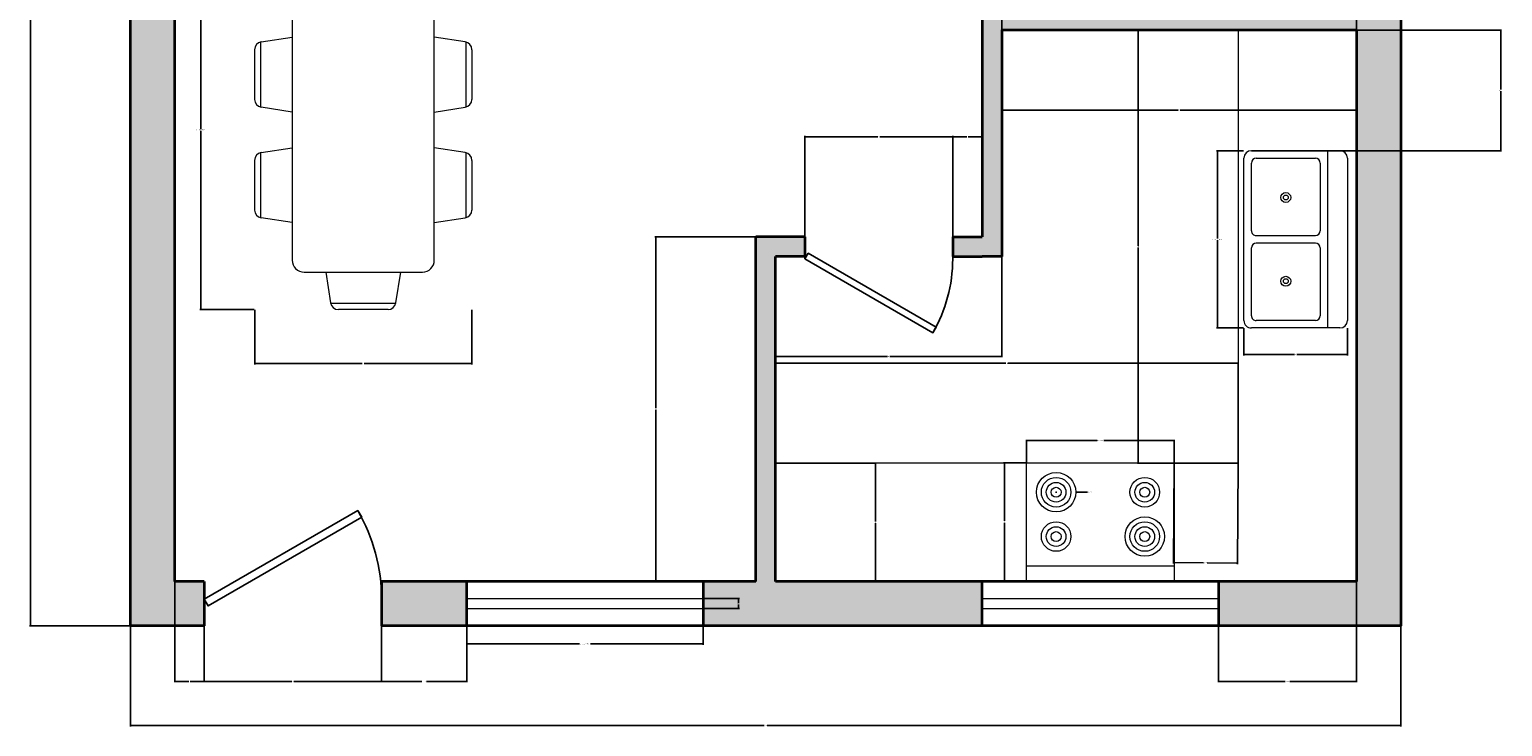
# Model space of a CAD drawing. Units: inches. Extents: x 1984 to 2284, y 2002 to 2421.
# Tile 1 of 4: x 1984 to 2284, y 2002 to 2144. Entities that reach past the tile are written whole.
import ezdxf

# ---------------------------------------------------------------- set-up
doc = ezdxf.new("R2010")
doc.units = ezdxf.units.IN
for name, color, linetype, lineweight in [('A-ANNO-DIMS', 2, 'Continuous', 18), ('A-DOOR', 3, 'Continuous', 25), ('A-EQPM', 9, 'Continuous', 18), ('A-FLOR-CASE', 9, 'Continuous', 20), ('A-FLOR-FIXT', 8, 'Continuous', 18), ('A-FURN', 8, 'Continuous', 18), ('A-GLAZ', 4, 'Continuous', 18), ('A-WALL', 7, 'Continuous', 35)]:
    doc.layers.add(name, color=color, linetype=linetype, lineweight=lineweight)
doc.layers.add('A-WALL-PATT', color=18, linetype='Continuous', lineweight=13, true_color=0x000000)
doc.styles.get("Standard").update_dxf_attribs({"font": 'arial.ttf'})
doc.dimstyles.get("Standard").update_dxf_attribs({"dimtxt": 0.18, "dimasz": 0.18, "dimexe": 0.18, "dimexo": 0.0625, "dimgap": 0.09, "dimtad": 0, "dimtih": 1, "dimtoh": 1, "dimdec": 4, "dimzin": 0, "dimdsep": 46, "dimtxsty": 'Standard', "dimcen": 0.09, "dimadec": 0, "dimazin": 0, "dimtfac": 1, "dimtdec": 4, "dimtofl": 0, "dimtmove": 0, "dimatfit": 3, "dimfxl": 1, "dimtolj": 1, "dimtzin": 0, "dimarcsym": 0})

# ---------------------------------------------------------------- blocks, each defined once
blk = doc.blocks.new('Range-Oven - 30 in top')
blk.add_line((0, -3), (30, -3))
blk.add_lwpolyline([(0, -24), (0, 0), (30, 0), (30, -24)], close=True)
for centre, radius in [((6, -9), 4), ((6, -9), 3), ((6, -9), 2), ((6, -9), 1), ((24, -9), 3), ((24, -9), 2), ((24, -9), 1), ((24, -18), 4), ((6, -18), 3), ((6, -18), 2), ((6, -18), 1), ((24, -18), 3), ((24, -18), 2), ((24, -18), 1)]:
    blk.add_circle(centre, radius)
blk = doc.blocks.new('Sink-double - 36 in top')
for p, q in [((-18, -4), (18, -4)), ((-0.75, -18.5), (-0.75, -6.5)), ((0.75, -6.5), (0.75, -18.5))]:
    blk.add_line(p, q)
for points in [[(-16.5, 0), (16.5, 0)], [(-18, -19.5), (-18, -1.5)], [(18, -1.5), (18, -19.5)], [(-15.5, -5.5), (-1.75, -5.5)], [(1.75, -5.5), (15.5, -5.5)], [(-16.5, -18.5), (-16.5, -6.5)], [(16.5, -6.5), (16.5, -18.5)], [(-1.75, -19.5), (-15.5, -19.5)], [(15.5, -19.5), (1.75, -19.5)], [(16.5, -21), (-16.5, -21)]]:
    blk.add_lwpolyline(points)
for centre, radius in [((-8.5, -12.5), 1), ((8.5, -12.5), 1), ((-8.5, -12.5), 0.5), ((8.5, -12.5), 0.5)]:
    blk.add_circle(centre, radius)
for centre, radius, start, end in [((-16.5, -1.5), 1.5, 90, 180), ((16.5, -1.5), 1.5, 0, 90), ((-15.5, -6.5), 1, 90, 180), ((-1.75, -6.5), 1, 0, 90), ((1.75, -6.5), 1, 90, 180), ((15.5, -6.5), 1, 0, 90), ((-16.5, -19.5), 1.5, 180, 270), ((-15.5, -18.5), 1, 180, 270), ((-1.75, -18.5), 1, 270, 0), ((1.75, -18.5), 1, 180, 270), ((15.5, -18.5), 1, 270, 0), ((16.5, -19.5), 1.5, 270, 0)]:
    blk.add_arc(centre, radius, start, end)
blk = doc.blocks.new('Dining Set - 36 x 72 in.')
for p, q in [((-20.29, 27.5), (-7.71, 27.5)), ((7.71, 27.5), (20.29, 27.5)), ((-22.26, 25.81), (-23.48, 18)), ((-22.23, 26), (-5.76, 26)), ((-4.52, 18), (-5.74, 25.81)), ((5.74, 25.81), (4.52, 18)), ((5.77, 26), (22.24, 26)), ((23.48, 18), (22.26, 25.81)), ((-36, 15), (-36, -15)), ((33, 18), (-33, 18)), ((36, -15), (36, 15)), ((-44, 8.23), (-44, -8.24)), ((-43.81, 8.26), (-36, 9.48)), ((43.81, 8.26), (36, 9.48)), ((44, 8.23), (44, -8.24)), ((-45.5, 6.29), (-45.5, -6.29)), ((45.5, 6.29), (45.5, -6.29)), ((-36, -9.48), (-43.81, -8.26)), ((36, -9.48), (43.81, -8.26)), ((-33, -18), (33, -18)), ((-22.26, -25.81), (-23.48, -18)), ((-4.52, -18), (-5.74, -25.81)), ((5.74, -25.81), (4.52, -18)), ((23.48, -18), (22.26, -25.81)), ((-22.23, -26), (-5.76, -26)), ((5.77, -26), (22.24, -26)), ((-20.29, -27.5), (-7.71, -27.5)), ((7.71, -27.5), (20.29, -27.5))]:
    blk.add_line(p, q)
for centre, radius, start, end in [((-20.29, 25.5), 2, 90, 171.1198), ((-7.71, 25.5), 2, 8.881, 90), ((7.71, 25.5), 2, 90, 171.1198), ((20.29, 25.5), 2, 8.881, 90), ((-33, 15), 3, 90, 180), ((33, 15), 3, 0, 90), ((-43.5, 6.29), 2, 98.8806, 180), ((43.5, 6.29), 2, 0, 81.1194), ((-43.5, -6.29), 2, 180, 261.1194), ((43.5, -6.29), 2, 278.8806, 0), ((-33, -15), 3, 180, 270), ((33, -15), 3, 270, 0), ((-20.29, -25.5), 2, 188.8802, 270), ((-7.71, -25.5), 2, 270, 351.1191), ((7.71, -25.5), 2, 188.8802, 270), ((20.29, -25.5), 2, 270, 351.1191)]:
    blk.add_arc(centre, radius, start, end)
blk = doc.blocks.new('*U10')
for p, q in [((0, 0), (0, -6)), ((40, 0), (40, -6))]:
    blk.add_line(p, q)
blk.add_lwpolyline([(0, 0), (34.64, 20), (35.52, 18.48), (0.87, -1.52)], close=True)
blk.add_arc((0, 0), 40, 0, 30)
blk = doc.blocks.new('*U11')
for p, q in [((0, 0), (0, 6)), ((40, 0), (40, 6))]:
    blk.add_line(p, q)
blk.add_lwpolyline([(0, 0), (34.64, -20), (35.52, -18.48), (0.87, 1.52)], close=True)
blk.add_arc((0, 0), 40, 330, 0)
blk = doc.blocks.new('GLAZING-48IN')
for p, q in [((0, 2), (48, 2)), ((0, 0), (48, 0))]:
    blk.add_line(p, q)
blk = doc.blocks.new('*D17')
at = {"layer": 'A-ANNO-DIMS', "color": 0, "lineweight": -2, "transparency": 16777216}
for p, q in [((2073.18, 2026.35), (2073.18, 2019.03)), ((2121.18, 2026.35), (2121.18, 2019.03)), ((2073.36, 2019.21), (2096.06, 2019.21)), ((2121, 2019.21), (2098.3, 2019.21))]:
    blk.add_line(p, q, dxfattribs=at)
at = {"layer": 'A-ANNO-DIMS', "color": 0, "transparency": 16777216}
for points in [[(2073.36, 2019.24), (2073.36, 2019.18), (2073.18, 2019.21)], [(2121, 2019.24), (2121, 2019.18), (2121.18, 2019.21)]]:
    blk.add_solid(points, dxfattribs=at)
at = {"layer": 'Defpoints', "color": 0, "transparency": 16777216}
for p in [(2073.18, 2026.41), (2121.18, 2026.41), (2121.18, 2019.21)]:
    blk.add_point(p, dxfattribs=at)
at = {"layer": 'A-ANNO-DIMS', "color": 0, "transparency": 16777216, "insert": (2097.18, 2019.21), "char_height": 0.18, "attachment_point": 5}
blk.add_mtext('\\A1;WINDOW 48 TYP.', dxfattribs=at)
blk = doc.blocks.new('*D18')
at = {"layer": 'A-ANNO-DIMS', "color": 0, "lineweight": -2, "transparency": 16777216}
for p, q in [((2121.24, 2028.41), (2128.56, 2028.41)), ((2121.24, 2026.41), (2128.56, 2026.41)), ((2128.38, 2028.23), (2128.38, 2027.59)), ((2128.38, 2026.59), (2128.38, 2027.23))]:
    blk.add_line(p, q, dxfattribs=at)
at = {"layer": 'A-ANNO-DIMS', "color": 0, "transparency": 16777216}
for points in [[(2128.35, 2028.23), (2128.41, 2028.23), (2128.38, 2028.41)], [(2128.35, 2026.59), (2128.41, 2026.59), (2128.38, 2026.41)]]:
    blk.add_solid(points, dxfattribs=at)
at = {"layer": 'Defpoints', "color": 0, "transparency": 16777216}
for p in [(2121.18, 2028.41), (2121.18, 2026.41), (2128.38, 2028.41)]:
    blk.add_point(p, dxfattribs=at)
at = {"layer": 'A-ANNO-DIMS', "color": 0, "transparency": 16777216, "insert": (2128.38, 2027.41), "char_height": 0.18, "attachment_point": 5}
blk.add_mtext('\\A1;2 TYP.', dxfattribs=at)
blk = doc.blocks.new('*D35')
at = {"layer": 'A-ANNO-DIMS', "color": 0, "lineweight": -2, "transparency": 16777216}
for p, q in [((2186.9, 2056.08), (2186.9, 2060.7)), ((2187.08, 2060.52), (2201.2, 2060.52)), ((2216.72, 2060.52), (2202.59, 2060.52)), ((2216.9, 2056.08), (2216.9, 2060.7))]:
    blk.add_line(p, q, dxfattribs=at)
at = {"layer": 'A-ANNO-DIMS', "color": 0, "transparency": 16777216}
for points in [[(2187.08, 2060.55), (2187.08, 2060.49), (2186.9, 2060.52)], [(2216.72, 2060.55), (2216.72, 2060.49), (2216.9, 2060.52)]]:
    blk.add_solid(points, dxfattribs=at)
at = {"layer": 'Defpoints', "color": 0, "transparency": 16777216}
for p in [(2186.9, 2060.52), (2186.9, 2056.02), (2216.9, 2056.02)]:
    blk.add_point(p, dxfattribs=at)
at = {"layer": 'A-ANNO-DIMS', "color": 0, "transparency": 16777216, "insert": (2201.9, 2060.52), "char_height": 0.18, "attachment_point": 5}
blk.add_mtext('\\A1;RANGE 30', dxfattribs=at)
blk = doc.blocks.new('*D36')
at = {"layer": 'A-ANNO-DIMS', "color": 0, "lineweight": -2, "transparency": 16777216}
for p, q in [((2186.83, 2056.02), (2182.22, 2056.02)), ((2182.4, 2055.84), (2182.4, 2044.2)), ((2182.4, 2032.2), (2182.4, 2043.84)), ((2186.83, 2032.02), (2182.22, 2032.02))]:
    blk.add_line(p, q, dxfattribs=at)
at = {"layer": 'A-ANNO-DIMS', "color": 0, "transparency": 16777216}
for points in [[(2182.37, 2055.84), (2182.43, 2055.84), (2182.4, 2056.02)], [(2182.37, 2032.2), (2182.43, 2032.2), (2182.4, 2032.02)]]:
    blk.add_solid(points, dxfattribs=at)
at = {"layer": 'Defpoints', "color": 0, "transparency": 16777216}
for p in [(2186.9, 2056.02), (2182.4, 2032.02), (2186.9, 2032.02)]:
    blk.add_point(p, dxfattribs=at)
at = {"layer": 'A-ANNO-DIMS', "color": 0, "transparency": 16777216, "insert": (2182.4, 2044.02), "char_height": 0.18, "attachment_point": 5}
blk.add_mtext('\\A1;24', dxfattribs=at)
blk = doc.blocks.new('*D37')
at = {"layer": 'A-ANNO-DIMS', "color": 0, "lineweight": -2, "transparency": 16777216}
for p, q in [((2230.98, 2119.39), (2225.46, 2119.39)), ((2225.64, 2119.21), (2225.64, 2101.57)), ((2225.64, 2083.57), (2225.64, 2101.2)), ((2230.98, 2083.39), (2225.46, 2083.39))]:
    blk.add_line(p, q, dxfattribs=at)
at = {"layer": 'A-ANNO-DIMS', "color": 0, "transparency": 16777216}
for points in [[(2225.61, 2119.21), (2225.67, 2119.21), (2225.64, 2119.39)], [(2225.61, 2083.57), (2225.67, 2083.57), (2225.64, 2083.39)]]:
    blk.add_solid(points, dxfattribs=at)
at = {"layer": 'Defpoints', "color": 0, "transparency": 16777216}
for p in [(2231.04, 2119.39), (2225.64, 2083.39), (2231.04, 2083.39)]:
    blk.add_point(p, dxfattribs=at)
at = {"layer": 'A-ANNO-DIMS', "color": 0, "transparency": 16777216, "insert": (2225.64, 2101.39), "char_height": 0.18, "attachment_point": 5}
blk.add_mtext('\\A1;DOUBLE SINK 36', dxfattribs=at)
blk = doc.blocks.new('*D38')
at = {"layer": 'A-ANNO-DIMS', "color": 0, "lineweight": -2, "transparency": 16777216}
for p, q in [((2231.04, 2083.32), (2231.04, 2077.81)), ((2252.04, 2083.32), (2252.04, 2077.81)), ((2231.22, 2077.99), (2241.34, 2077.99)), ((2251.86, 2077.99), (2241.75, 2077.99))]:
    blk.add_line(p, q, dxfattribs=at)
at = {"layer": 'A-ANNO-DIMS', "color": 0, "transparency": 16777216}
for points in [[(2231.22, 2078.02), (2231.22, 2077.96), (2231.04, 2077.99)], [(2251.86, 2078.02), (2251.86, 2077.96), (2252.04, 2077.99)]]:
    blk.add_solid(points, dxfattribs=at)
at = {"layer": 'Defpoints', "color": 0, "transparency": 16777216}
for p in [(2231.04, 2083.39), (2252.04, 2083.39), (2252.04, 2077.99)]:
    blk.add_point(p, dxfattribs=at)
at = {"layer": 'A-ANNO-DIMS', "color": 0, "transparency": 16777216, "insert": (2241.54, 2077.99), "char_height": 0.18, "attachment_point": 5}
blk.add_mtext('\\A1;21', dxfattribs=at)
blk = doc.blocks.new('*D39')
at = {"layer": 'A-ANNO-DIMS', "color": 0, "lineweight": -2, "transparency": 16777216}
for p, q in [((2030.05, 2160.11), (2018.99, 2160.11)), ((2019.17, 2159.93), (2019.17, 2123.8)), ((2019.17, 2087.31), (2019.17, 2123.44)), ((2030.05, 2087.13), (2018.99, 2087.13))]:
    blk.add_line(p, q, dxfattribs=at)
at = {"layer": 'A-ANNO-DIMS', "color": 0, "transparency": 16777216}
for points in [[(2019.14, 2159.93), (2019.2, 2159.93), (2019.17, 2160.11)], [(2019.14, 2087.31), (2019.2, 2087.31), (2019.17, 2087.13)]]:
    blk.add_solid(points, dxfattribs=at)
at = {"layer": 'Defpoints', "color": 0, "transparency": 16777216}
for p in [(2030.12, 2160.11), (2019.17, 2087.13), (2030.12, 2087.13)]:
    blk.add_point(p, dxfattribs=at)
at = {"layer": 'A-ANNO-DIMS', "color": 0, "transparency": 16777216, "insert": (2019.17, 2123.62), "char_height": 0.18, "attachment_point": 5}
blk.add_mtext('\\A1;DINING SET 73', dxfattribs=at)
blk = doc.blocks.new('*D40')
at = {"layer": 'A-ANNO-DIMS', "color": 0, "lineweight": -2, "transparency": 16777216}
for p, q in [((2030.12, 2087.07), (2030.12, 2076)), ((2074.23, 2087.07), (2074.23, 2076)), ((2030.3, 2076.18), (2051.95, 2076.18)), ((2074.05, 2076.18), (2052.39, 2076.18))]:
    blk.add_line(p, q, dxfattribs=at)
at = {"layer": 'A-ANNO-DIMS', "color": 0, "transparency": 16777216}
for points in [[(2030.3, 2076.21), (2030.3, 2076.15), (2030.12, 2076.18)], [(2074.05, 2076.21), (2074.05, 2076.15), (2074.23, 2076.18)]]:
    blk.add_solid(points, dxfattribs=at)
at = {"layer": 'Defpoints', "color": 0, "transparency": 16777216}
for p in [(2030.12, 2087.13), (2074.23, 2087.13), (2074.23, 2076.18)]:
    blk.add_point(p, dxfattribs=at)
at = {"layer": 'A-ANNO-DIMS', "color": 0, "transparency": 16777216, "insert": (2052.17, 2076.18), "char_height": 0.18, "attachment_point": 5}
blk.add_mtext('\\A1;44', dxfattribs=at)
blk = doc.blocks.new('*D41')
at = {"layer": 'A-ANNO-DIMS', "color": 0, "lineweight": -2, "transparency": 16777216}
for p, q in [((2004.89, 2022.85), (2004.89, 2002.43)), ((2262.89, 2022.85), (2262.89, 2002.43)), ((2005.07, 2002.61), (2133.59, 2002.61)), ((2262.71, 2002.61), (2134.18, 2002.61))]:
    blk.add_line(p, q, dxfattribs=at)
at = {"layer": 'A-ANNO-DIMS', "color": 0, "transparency": 16777216}
for points in [[(2005.07, 2002.64), (2005.07, 2002.58), (2004.89, 2002.61)], [(2262.71, 2002.64), (2262.71, 2002.58), (2262.89, 2002.61)]]:
    blk.add_solid(points, dxfattribs=at)
at = {"layer": 'Defpoints', "color": 0, "transparency": 16777216}
for p in [(2004.89, 2022.91), (2262.89, 2022.91), (2262.89, 2002.61)]:
    blk.add_point(p, dxfattribs=at)
at = {"layer": 'A-ANNO-DIMS', "color": 0, "transparency": 16777216, "insert": (2133.89, 2002.61), "char_height": 0.18, "attachment_point": 5}
blk.add_mtext('\\A1;258', dxfattribs=at)
blk = doc.blocks.new('*D42')
at = {"layer": 'A-ANNO-DIMS', "color": 0, "lineweight": -2, "transparency": 16777216}
for p, q in [((2004.82, 2400.91), (1984.41, 2400.91)), ((1984.59, 2400.73), (1984.59, 2212.09)), ((1984.59, 2023.09), (1984.59, 2211.73)), ((2004.82, 2022.91), (1984.41, 2022.91))]:
    blk.add_line(p, q, dxfattribs=at)
at = {"layer": 'A-ANNO-DIMS', "color": 0, "transparency": 16777216}
for points in [[(1984.56, 2400.73), (1984.62, 2400.73), (1984.59, 2400.91)], [(1984.56, 2023.09), (1984.62, 2023.09), (1984.59, 2022.91)]]:
    blk.add_solid(points, dxfattribs=at)
at = {"layer": 'Defpoints', "color": 0, "transparency": 16777216}
for p in [(1984.59, 2400.91), (2004.89, 2400.91), (2004.89, 2022.91)]:
    blk.add_point(p, dxfattribs=at)
at = {"layer": 'A-ANNO-DIMS', "color": 0, "transparency": 16777216, "insert": (1984.59, 2211.91), "char_height": 0.18, "attachment_point": 5}
blk.add_mtext('\\A1;378', dxfattribs=at)
blk = doc.blocks.new('*D53')
at = {"layer": 'A-ANNO-DIMS', "color": 0, "lineweight": -2, "transparency": 16777216}
for p, q in [((2229.82, 2143.91), (2209.41, 2143.91)), ((2209.59, 2143.73), (2209.59, 2100.09)), ((2209.59, 2056.09), (2209.59, 2099.73)), ((2229.82, 2055.91), (2209.41, 2055.91))]:
    blk.add_line(p, q, dxfattribs=at)
at = {"layer": 'A-ANNO-DIMS', "color": 0, "transparency": 16777216}
for points in [[(2209.56, 2143.73), (2209.62, 2143.73), (2209.59, 2143.91)], [(2209.56, 2056.09), (2209.62, 2056.09), (2209.59, 2055.91)]]:
    blk.add_solid(points, dxfattribs=at)
at = {"layer": 'Defpoints', "color": 0, "transparency": 16777216}
for p in [(2209.59, 2143.91), (2229.89, 2143.91), (2229.89, 2055.91)]:
    blk.add_point(p, dxfattribs=at)
at = {"layer": 'A-ANNO-DIMS', "color": 0, "transparency": 16777216, "insert": (2209.59, 2099.91), "char_height": 0.18, "attachment_point": 5}
blk.add_mtext('\\A1;88', dxfattribs=at)
blk = doc.blocks.new('*D54')
at = {"layer": 'A-ANNO-DIMS', "color": 0, "lineweight": -2, "transparency": 16777216}
for p, q in [((2181.89, 2147.85), (2181.89, 2127.43)), ((2253.89, 2147.85), (2253.89, 2127.43)), ((2182.07, 2127.61), (2217.67, 2127.61)), ((2253.71, 2127.61), (2218.1, 2127.61))]:
    blk.add_line(p, q, dxfattribs=at)
at = {"layer": 'A-ANNO-DIMS', "color": 0, "transparency": 16777216}
for points in [[(2182.07, 2127.64), (2182.07, 2127.58), (2181.89, 2127.61)], [(2253.71, 2127.64), (2253.71, 2127.58), (2253.89, 2127.61)]]:
    blk.add_solid(points, dxfattribs=at)
at = {"layer": 'Defpoints', "color": 0, "transparency": 16777216}
for p in [(2181.89, 2147.91), (2253.89, 2147.91), (2181.89, 2127.61)]:
    blk.add_point(p, dxfattribs=at)
at = {"layer": 'A-ANNO-DIMS', "color": 0, "transparency": 16777216, "insert": (2217.89, 2127.61), "char_height": 0.18, "attachment_point": 5}
blk.add_mtext('\\A1;72', dxfattribs=at)
blk = doc.blocks.new('*D55')
at = {"layer": 'A-ANNO-DIMS', "color": 0, "lineweight": -2, "transparency": 16777216}
for p, q in [((2131.82, 2101.91), (2111.41, 2101.91)), ((2111.59, 2101.73), (2111.59, 2067.09)), ((2111.59, 2032.09), (2111.59, 2066.73)), ((2131.82, 2031.91), (2111.41, 2031.91))]:
    blk.add_line(p, q, dxfattribs=at)
at = {"layer": 'A-ANNO-DIMS', "color": 0, "transparency": 16777216}
for points in [[(2111.56, 2101.73), (2111.62, 2101.73), (2111.59, 2101.91)], [(2111.56, 2032.09), (2111.62, 2032.09), (2111.59, 2031.91)]]:
    blk.add_solid(points, dxfattribs=at)
at = {"layer": 'Defpoints', "color": 0, "transparency": 16777216}
for p in [(2111.59, 2101.91), (2131.89, 2101.91), (2131.89, 2031.91)]:
    blk.add_point(p, dxfattribs=at)
at = {"layer": 'A-ANNO-DIMS', "color": 0, "transparency": 16777216, "insert": (2111.59, 2066.91), "char_height": 0.18, "attachment_point": 5}
blk.add_mtext('\\A1;70', dxfattribs=at)
blk = doc.blocks.new('*D56')
at = {"layer": 'A-ANNO-DIMS', "color": 0, "lineweight": -2, "transparency": 16777216}
for p, q in [((2135.89, 2097.85), (2135.89, 2077.43)), ((2181.89, 2097.85), (2181.89, 2077.43)), ((2136.07, 2077.61), (2158.66, 2077.61)), ((2181.71, 2077.61), (2159.11, 2077.61))]:
    blk.add_line(p, q, dxfattribs=at)
at = {"layer": 'A-ANNO-DIMS', "color": 0, "transparency": 16777216}
for points in [[(2136.07, 2077.64), (2136.07, 2077.58), (2135.89, 2077.61)], [(2181.71, 2077.64), (2181.71, 2077.58), (2181.89, 2077.61)]]:
    blk.add_solid(points, dxfattribs=at)
at = {"layer": 'Defpoints', "color": 0, "transparency": 16777216}
for p in [(2135.89, 2097.91), (2181.89, 2097.91), (2135.89, 2077.61)]:
    blk.add_point(p, dxfattribs=at)
at = {"layer": 'A-ANNO-DIMS', "color": 0, "transparency": 16777216, "insert": (2158.89, 2077.61), "char_height": 0.18, "attachment_point": 5}
blk.add_mtext('\\A1;46', dxfattribs=at)
blk = doc.blocks.new('*D57')
at = {"layer": 'A-ANNO-DIMS', "color": 0, "lineweight": -2, "transparency": 16777216}
for p, q in [((2019.89, 2031.85), (2019.89, 2011.43)), ((2055.89, 2031.85), (2055.89, 2011.43)), ((2020.07, 2011.61), (2037.67, 2011.61)), ((2055.71, 2011.61), (2038.1, 2011.61))]:
    blk.add_line(p, q, dxfattribs=at)
at = {"layer": 'A-ANNO-DIMS', "color": 0, "transparency": 16777216}
for points in [[(2020.07, 2011.64), (2020.07, 2011.58), (2019.89, 2011.61)], [(2055.71, 2011.64), (2055.71, 2011.58), (2055.89, 2011.61)]]:
    blk.add_solid(points, dxfattribs=at)
at = {"layer": 'Defpoints', "color": 0, "transparency": 16777216}
for p in [(2019.89, 2031.91), (2055.89, 2031.91), (2019.89, 2011.61)]:
    blk.add_point(p, dxfattribs=at)
at = {"layer": 'A-ANNO-DIMS', "color": 0, "transparency": 16777216, "insert": (2037.89, 2011.61), "char_height": 0.18, "attachment_point": 5}
blk.add_mtext('\\A1;36', dxfattribs=at)
blk = doc.blocks.new('*D58')
at = {"layer": 'A-ANNO-DIMS', "color": 0, "lineweight": -2, "transparency": 16777216}
for p, q in [((2013.89, 2031.85), (2013.89, 2011.43)), ((2019.89, 2031.85), (2019.89, 2011.43)), ((2014.07, 2011.61), (2016.74, 2011.61)), ((2019.71, 2011.61), (2017.03, 2011.61))]:
    blk.add_line(p, q, dxfattribs=at)
at = {"layer": 'A-ANNO-DIMS', "color": 0, "transparency": 16777216}
for points in [[(2014.07, 2011.64), (2014.07, 2011.58), (2013.89, 2011.61)], [(2019.71, 2011.64), (2019.71, 2011.58), (2019.89, 2011.61)]]:
    blk.add_solid(points, dxfattribs=at)
at = {"layer": 'Defpoints', "color": 0, "transparency": 16777216}
for p in [(2013.89, 2031.91), (2019.89, 2031.91), (2013.89, 2011.61)]:
    blk.add_point(p, dxfattribs=at)
at = {"layer": 'A-ANNO-DIMS', "color": 0, "transparency": 16777216, "insert": (2016.89, 2011.61), "char_height": 0.18, "attachment_point": 5}
blk.add_mtext('\\A1;6', dxfattribs=at)
blk = doc.blocks.new('*D59')
at = {"layer": 'A-ANNO-DIMS', "color": 0, "lineweight": -2, "transparency": 16777216}
for p, q in [((2055.89, 2031.85), (2055.89, 2011.43)), ((2073.18, 2031.85), (2073.18, 2011.43)), ((2056.07, 2011.61), (2064.08, 2011.61)), ((2073, 2011.61), (2064.99, 2011.61))]:
    blk.add_line(p, q, dxfattribs=at)
at = {"layer": 'A-ANNO-DIMS', "color": 0, "transparency": 16777216}
for points in [[(2056.07, 2011.64), (2056.07, 2011.58), (2055.89, 2011.61)], [(2073, 2011.64), (2073, 2011.58), (2073.18, 2011.61)]]:
    blk.add_solid(points, dxfattribs=at)
at = {"layer": 'Defpoints', "color": 0, "transparency": 16777216}
for p in [(2055.89, 2031.91), (2073.18, 2031.91), (2055.89, 2011.61)]:
    blk.add_point(p, dxfattribs=at)
at = {"layer": 'A-ANNO-DIMS', "color": 0, "transparency": 16777216, "insert": (2064.53, 2011.61), "char_height": 0.18, "attachment_point": 5}
blk.add_mtext('\\A1;17.293', dxfattribs=at)
blk = doc.blocks.new('*D60')
at = {"layer": 'A-ANNO-DIMS', "color": 0, "lineweight": -2, "transparency": 16777216}
for p, q in [((2225.9, 2031.85), (2225.9, 2011.43)), ((2253.89, 2031.85), (2253.89, 2011.43)), ((2226.08, 2011.61), (2239.43, 2011.61)), ((2253.71, 2011.61), (2240.36, 2011.61))]:
    blk.add_line(p, q, dxfattribs=at)
at = {"layer": 'A-ANNO-DIMS', "color": 0, "transparency": 16777216}
for points in [[(2226.08, 2011.64), (2226.08, 2011.58), (2225.9, 2011.61)], [(2253.71, 2011.64), (2253.71, 2011.58), (2253.89, 2011.61)]]:
    blk.add_solid(points, dxfattribs=at)
at = {"layer": 'Defpoints', "color": 0, "transparency": 16777216}
for p in [(2225.9, 2031.91), (2253.89, 2031.91), (2225.9, 2011.61)]:
    blk.add_point(p, dxfattribs=at)
at = {"layer": 'A-ANNO-DIMS', "color": 0, "transparency": 16777216, "insert": (2239.89, 2011.61), "char_height": 0.18, "attachment_point": 5}
blk.add_mtext('\\A1;27.987', dxfattribs=at)
blk = doc.blocks.new('*D67')
at = {"layer": 'A-ANNO-DIMS', "color": 0, "lineweight": -2, "transparency": 16777216}
for p, q in [((2141.89, 2101.97), (2141.89, 2122.39)), ((2142.07, 2122.21), (2156.67, 2122.21)), ((2171.71, 2122.21), (2157.1, 2122.21)), ((2171.89, 2101.97), (2171.89, 2122.39))]:
    blk.add_line(p, q, dxfattribs=at)
at = {"layer": 'A-ANNO-DIMS', "color": 0, "transparency": 16777216}
for points in [[(2142.07, 2122.24), (2142.07, 2122.18), (2141.89, 2122.21)], [(2171.71, 2122.24), (2171.71, 2122.18), (2171.89, 2122.21)]]:
    blk.add_solid(points, dxfattribs=at)
at = {"layer": 'Defpoints', "color": 0, "transparency": 16777216}
for p in [(2171.89, 2122.21), (2141.89, 2101.91), (2171.89, 2101.91)]:
    blk.add_point(p, dxfattribs=at)
at = {"layer": 'A-ANNO-DIMS', "color": 0, "transparency": 16777216, "insert": (2156.89, 2122.21), "char_height": 0.18, "attachment_point": 5}
blk.add_mtext('\\A1;30', dxfattribs=at)
blk = doc.blocks.new('*D68')
at = {"layer": 'A-ANNO-DIMS', "color": 0, "lineweight": -2, "transparency": 16777216}
for p, q in [((2171.89, 2101.97), (2171.89, 2122.39)), ((2172.07, 2122.21), (2174.74, 2122.21)), ((2177.71, 2122.21), (2175.03, 2122.21)), ((2177.89, 2101.97), (2177.89, 2122.39))]:
    blk.add_line(p, q, dxfattribs=at)
at = {"layer": 'A-ANNO-DIMS', "color": 0, "transparency": 16777216}
for points in [[(2172.07, 2122.24), (2172.07, 2122.18), (2171.89, 2122.21)], [(2177.71, 2122.24), (2177.71, 2122.18), (2177.89, 2122.21)]]:
    blk.add_solid(points, dxfattribs=at)
at = {"layer": 'Defpoints', "color": 0, "transparency": 16777216}
for p in [(2177.89, 2122.21), (2171.89, 2101.91), (2177.89, 2101.91)]:
    blk.add_point(p, dxfattribs=at)
at = {"layer": 'A-ANNO-DIMS', "color": 0, "transparency": 16777216, "insert": (2174.89, 2122.21), "char_height": 0.18, "attachment_point": 5}
blk.add_mtext('\\A1;6', dxfattribs=at)
blk = doc.blocks.new('*D73')
at = {"layer": 'A-ANNO-DIMS', "color": 0, "lineweight": -2, "transparency": 16777216}
for p, q in [((2216.9, 2055.96), (2216.72, 2035.54)), ((2229.88, 2055.85), (2229.71, 2035.43)), ((2216.9, 2035.72), (2222.83, 2035.67)), ((2229.53, 2035.61), (2223.6, 2035.66))]:
    blk.add_line(p, q, dxfattribs=at)
at = {"layer": 'A-ANNO-DIMS', "color": 0, "transparency": 16777216}
for points in [[(2216.9, 2035.75), (2216.9, 2035.69), (2216.72, 2035.72)], [(2229.53, 2035.64), (2229.53, 2035.58), (2229.71, 2035.61)]]:
    blk.add_solid(points, dxfattribs=at)
at = {"layer": 'Defpoints', "color": 0, "transparency": 16777216}
for p in [(2216.9, 2056.02), (2229.89, 2055.91), (2216.72, 2035.72)]:
    blk.add_point(p, dxfattribs=at)
at = {"layer": 'A-ANNO-DIMS', "color": 0, "transparency": 16777216, "insert": (2223.22, 2035.67), "char_height": 0.18, "attachment_point": 5}
blk.add_mtext('\\A1;12.99', dxfattribs=at)
blk = doc.blocks.new('*D74')
at = {"layer": 'A-ANNO-DIMS', "color": 0, "lineweight": -2, "transparency": 16777216}
for p, q in [((2135.95, 2055.91), (2156.37, 2055.91)), ((2156.19, 2055.73), (2156.19, 2044.09)), ((2156.19, 2032.09), (2156.19, 2043.73)), ((2135.95, 2031.91), (2156.37, 2031.91))]:
    blk.add_line(p, q, dxfattribs=at)
at = {"layer": 'A-ANNO-DIMS', "color": 0, "transparency": 16777216}
for points in [[(2156.16, 2055.73), (2156.22, 2055.73), (2156.19, 2055.91)], [(2156.16, 2032.09), (2156.22, 2032.09), (2156.19, 2031.91)]]:
    blk.add_solid(points, dxfattribs=at)
at = {"layer": 'Defpoints', "color": 0, "transparency": 16777216}
for p in [(2135.89, 2055.91), (2135.89, 2031.91), (2156.19, 2031.91)]:
    blk.add_point(p, dxfattribs=at)
at = {"layer": 'A-ANNO-DIMS', "color": 0, "transparency": 16777216, "insert": (2156.19, 2043.91), "char_height": 0.18, "attachment_point": 5}
blk.add_mtext('\\A1;24', dxfattribs=at)
blk = doc.blocks.new('*D75')
at = {"layer": 'A-ANNO-DIMS', "color": 0, "lineweight": -2, "transparency": 16777216}
for p, q in [((2135.89, 2055.97), (2135.89, 2076.39)), ((2229.89, 2055.97), (2229.89, 2076.39)), ((2136.07, 2076.21), (2182.67, 2076.21)), ((2229.71, 2076.21), (2183.1, 2076.21))]:
    blk.add_line(p, q, dxfattribs=at)
at = {"layer": 'A-ANNO-DIMS', "color": 0, "transparency": 16777216}
for points in [[(2136.07, 2076.24), (2136.07, 2076.18), (2135.89, 2076.21)], [(2229.71, 2076.24), (2229.71, 2076.18), (2229.89, 2076.21)]]:
    blk.add_solid(points, dxfattribs=at)
at = {"layer": 'Defpoints', "color": 0, "transparency": 16777216}
for p in [(2229.89, 2076.21), (2135.89, 2055.91), (2229.89, 2055.91)]:
    blk.add_point(p, dxfattribs=at)
at = {"layer": 'A-ANNO-DIMS', "color": 0, "transparency": 16777216, "insert": (2182.89, 2076.21), "char_height": 0.18, "attachment_point": 5}
blk.add_mtext('\\A1;94', dxfattribs=at)
blk = doc.blocks.new('*D76')
at = {"layer": 'A-ANNO-DIMS', "color": 0, "lineweight": -2, "transparency": 16777216}
for p, q in [((2229.95, 2143.91), (2283.37, 2143.91)), ((2283.19, 2143.73), (2283.19, 2131.83)), ((2283.19, 2119.57), (2283.19, 2131.47)), ((2232.61, 2119.39), (2283.37, 2119.39))]:
    blk.add_line(p, q, dxfattribs=at)
at = {"layer": 'A-ANNO-DIMS', "color": 0, "transparency": 16777216}
for points in [[(2283.16, 2143.73), (2283.22, 2143.73), (2283.19, 2143.91)], [(2283.16, 2119.57), (2283.22, 2119.57), (2283.19, 2119.39)]]:
    blk.add_solid(points, dxfattribs=at)
at = {"layer": 'Defpoints', "color": 0, "transparency": 16777216}
for p in [(2229.89, 2143.91), (2283.19, 2143.91), (2232.54, 2119.39)]:
    blk.add_point(p, dxfattribs=at)
at = {"layer": 'A-ANNO-DIMS', "color": 0, "transparency": 16777216, "insert": (2283.19, 2131.65), "char_height": 0.18, "attachment_point": 5}
blk.add_mtext('\\A1;24.525', dxfattribs=at)
blk = doc.blocks.new('*D82')
at = {"layer": 'A-ANNO-DIMS', "color": 0, "lineweight": -2, "transparency": 16777216}
for p, q in [((2192.81, 2050.02), (2192.99, 2050.02)), ((2192.9, 2049.93), (2192.9, 2050.11)), ((2199.3, 2050.02), (2197.08, 2050.02))]:
    blk.add_line(p, q, dxfattribs=at)
at = {"layer": 'A-ANNO-DIMS', "color": 0, "transparency": 16777216}
blk.add_solid([(2197.08, 2050.05), (2197.08, 2049.99), (2196.9, 2050.02)], dxfattribs=at)
at = {"layer": 'Defpoints', "color": 0, "transparency": 16777216}
for p in [(2188.9, 2050.02), (2196.9, 2050.02)]:
    blk.add_point(p, dxfattribs=at)
at = {"layer": 'A-ANNO-DIMS', "color": 0, "transparency": 16777216, "insert": (2199.73, 2050.02), "char_height": 0.18, "attachment_point": 5}
blk.add_mtext('\\A1;2X ∅8', dxfattribs=at)

msp = doc.modelspace()

# ---------------------------------------------------------------- hatches: boundary and pattern name
at = {"layer": 'A-WALL-PATT'}
h = msp.add_hatch(color=256, dxfattribs=at)
h.dxf.hatch_style = 1
h.paths.add_polyline_path([(2052.8198, 2400.9122), (2004.8852, 2400.9122), (2004.8852, 2022.9122), (2019.8852, 2022.9122), (2019.8852, 2031.9122), (2013.8852, 2031.9122), (2013.8852, 2267.9122), (2095.8852, 2267.9122), (2095.8852, 2271.9122), (2013.8852, 2271.9122), (2013.8852, 2391.9122), (2052.8198, 2391.9122)])
h = msp.add_hatch(color=256, dxfattribs=at)
h.dxf.hatch_style = 1
h.paths.add_polyline_path([(2262.8852, 2161.8141), (2253.8852, 2161.8141), (2253.8852, 2147.9122), (2181.8852, 2147.9122), (2181.8852, 2163.9122), (2177.8852, 2163.9122), (2177.8852, 2147.9122), (2177.8852, 2101.9122), (2171.8852, 2101.9122), (2171.8852, 2097.9122), (2177.8852, 2097.9122), (2181.8852, 2097.9122), (2181.8852, 2143.9122), (2253.8852, 2143.9122), (2253.8852, 2031.9122), (2225.8984, 2031.9122), (2225.8984, 2022.9122), (2262.8852, 2022.9122)])
h = msp.add_hatch(color=256, dxfattribs=at)
h.dxf.hatch_style = 1
h.paths.add_polyline_path([(2177.8984, 2031.9122), (2135.8852, 2031.9122), (2135.8852, 2097.9122), (2141.8852, 2097.9122), (2141.8852, 2101.9122), (2131.8852, 2101.9122), (2131.8852, 2031.9122), (2121.1786, 2031.9122), (2121.1786, 2022.9122), (2177.8984, 2022.9122)])
h = msp.add_hatch(color=256, dxfattribs=at)
h.dxf.hatch_style = 1
h.paths.add_polyline_path([(2073.1786, 2031.9122), (2055.8852, 2031.9122), (2055.8852, 2022.9122), (2073.1786, 2022.9122)])

# ---------------------------------------------------------------- linework, layer by layer
at = {"layer": 'A-FLOR-CASE'}
for p, q in [((2229.8852, 2143.9122), (2229.8852, 2055.9122)), ((2229.8852, 2055.9122), (2135.8852, 2055.9122))]:
    msp.add_line(p, q, dxfattribs=at)
at = {"layer": 'A-WALL'}
for p, q in [((2013.8852, 2031.9122), (2013.8852, 2267.9122)), ((2177.8852, 2147.9122), (2177.8852, 2101.9122)), ((2177.8852, 2143.9122), (2177.8852, 2101.9122)), ((2181.8852, 2143.9122), (2253.8852, 2143.9122)), ((2181.8852, 2143.9122), (2181.8852, 2097.9122)), ((2253.8852, 2143.9122), (2253.8852, 2031.9122)), ((2131.8852, 2031.9122), (2131.8852, 2101.9122)), ((2141.8852, 2101.9122), (2131.8852, 2101.9122)), ((2141.8852, 2101.9122), (2141.8852, 2097.9122)), ((2171.8852, 2101.9122), (2171.8852, 2097.9122)), ((2171.8852, 2101.9122), (2177.8852, 2101.9122)), ((2135.8852, 2031.9122), (2135.8852, 2097.9122)), ((2141.8852, 2097.9122), (2135.8852, 2097.9122)), ((2171.8852, 2097.9122), (2177.8852, 2097.9122)), ((2181.8852, 2097.9122), (2177.8852, 2097.9122)), ((2019.8852, 2031.9122), (2013.8852, 2031.9122)), ((2019.8852, 2031.9122), (2019.8852, 2022.9122)), ((2131.8852, 2031.9122), (2055.8852, 2031.9122)), ((2055.8852, 2031.9122), (2055.8852, 2022.9122)), ((2253.8852, 2031.9122), (2135.8852, 2031.9122))]:
    msp.add_line(p, q, dxfattribs=at)
for points in [[(2019.8852, 2022.9122), (2004.8852, 2022.9122), (2004.8852, 2400.9122), (2262.8852, 2400.9122), (2262.8852, 2022.9122), (2055.8852, 2022.9122)], [(2073.1786, 2022.9122), (2073.1786, 2031.9122)], [(2121.1786, 2031.9122), (2121.1786, 2022.9122)], [(2177.8984, 2022.9122), (2177.8984, 2031.9122)], [(2225.8984, 2031.9122), (2225.8984, 2022.9122)]]:
    msp.add_lwpolyline(points, dxfattribs=at)

# ---------------------------------------------------------------- block references
at = {"layer": 'A-DOOR'}
for name, p, xscale, yscale, zscale in [('*U11', (2141.8852, 2097.4122), 0.75, 0.75, 0.75), ('*U10', (2019.8852, 2028.3122), 0.9, 0.9, 0.9)]:
    msp.add_blockref(name, p, dxfattribs=dict(at, xscale=xscale, yscale=yscale, zscale=zscale))
at = {"layer": 'A-EQPM', "rotation": 180}
msp.add_blockref('Range-Oven - 30 in top', (2216.8965, 2032.0222), dxfattribs=at)
at = {"layer": 'A-FLOR-FIXT', "rotation": 270}
msp.add_blockref('Sink-double - 36 in top', (2252.0426, 2101.3872), dxfattribs=at)
at = {"layer": 'A-FURN', "xscale": 0.8020426707360627, "yscale": 0.8020426707360627, "zscale": 0.8020426707360627, "rotation": 270}
msp.add_blockref('Dining Set - 36 x 72 in.', (2052.1712, 2123.6218), dxfattribs=at)
at = {"layer": 'A-GLAZ'}
for p in [(2073.1786, 2026.4122), (2177.8984, 2026.4122)]:
    msp.add_blockref('GLAZING-48IN', p, dxfattribs=at)

# ---------------------------------------------------------------- dimensions: what is measured, and where the dimension line sits
at = {"layer": 'A-ANNO-DIMS'}
for base, p1, p2, angle, override, picture, middle in [((1984.5852, 2400.9122), (2004.8852, 2022.9122), (2004.8852, 2400.9122), 90, {"dimdec": 0, "dimlfac": 1, "dimrnd": 0, "dimzin": 0, "dimdsep": 46, "dimlunit": 2}, '*D42', (1984.5852, 2211.9122)), ((2181.8852, 2127.6122), (2253.8852, 2147.9122), (2181.8852, 2147.9122), 180, {"dimdec": 0, "dimlfac": 1, "dimrnd": 0, "dimzin": 0, "dimdsep": 46, "dimlunit": 2}, '*D54', (2217.8852, 2127.6122)), ((2209.5852, 2143.9122), (2229.8852, 2055.9122), (2229.8852, 2143.9122), 90, {"dimdec": 0, "dimlfac": 1, "dimrnd": 0, "dimzin": 0, "dimdsep": 46, "dimlunit": 2}, '*D53', (2209.5852, 2099.9122)), ((2283.1852, 2143.9122), (2232.5426, 2119.3872), (2229.8852, 2143.9122), 90, {"dimdec": 3, "dimlfac": 1, "dimrnd": 0, "dimzin": 0, "dimdsep": 46, "dimlunit": 2}, '*D76', (2283.1852, 2131.6497)), ((2111.5852, 2101.9122), (2131.8852, 2031.9122), (2131.8852, 2101.9122), 90, {"dimdec": 0, "dimlfac": 1, "dimrnd": 0, "dimzin": 0, "dimdsep": 46, "dimlunit": 2}, '*D55', (2111.5852, 2066.9122)), ((2135.8852, 2077.6122), (2181.8852, 2097.9122), (2135.8852, 2097.9122), 180, {"dimdec": 0, "dimlfac": 1, "dimrnd": 0, "dimzin": 0, "dimdsep": 46, "dimlunit": 2}, '*D56', (2158.8852, 2077.6122)), ((2156.1852, 2031.9122), (2135.8852, 2055.9122), (2135.8852, 2031.9122), 270, {"dimdec": 0, "dimlfac": 1, "dimrnd": 0, "dimzin": 0, "dimdsep": 46, "dimlunit": 2}, '*D74', (2156.1852, 2043.9122)), ((2182.3965, 2032.0222), (2186.8965, 2056.0222), (2186.8965, 2032.0222), 270, {"dimdec": 0, "dimlfac": 1, "dimrnd": 0, "dimzin": 0, "dimdsep": 46, "dimlunit": 2}, '*D36', (2182.3965, 2044.0222)), ((2216.7246, 2035.7229), (2229.8852, 2055.9122), (2216.8965, 2056.0222), 179.514878, {"dimdec": 2, "dimlfac": 1, "dimrnd": 0, "dimzin": 0, "dimdsep": 46, "dimlunit": 2}, '*D73', (2223.219, 2035.6679)), ((2013.8852, 2011.6122), (2019.8852, 2031.9122), (2013.8852, 2031.9122), 180, {"dimdec": 0, "dimlfac": 1, "dimrnd": 0, "dimzin": 0, "dimdsep": 46, "dimlunit": 2}, '*D58', (2016.8852, 2011.6122)), ((2019.8852, 2011.6122), (2055.8852, 2031.9122), (2019.8852, 2031.9122), 180, {"dimdec": 0, "dimlfac": 1, "dimrnd": 0, "dimzin": 0, "dimdsep": 46, "dimlunit": 2}, '*D57', (2037.8852, 2011.6122)), ((2055.8852, 2011.6122), (2073.1786, 2031.9122), (2055.8852, 2031.9122), 180, {"dimdec": 3, "dimlfac": 1, "dimrnd": 0, "dimzin": 0, "dimdsep": 46, "dimlunit": 2}, '*D59', (2064.5319, 2011.6122)), ((2225.8984, 2011.6122), (2253.8852, 2031.9122), (2225.8984, 2031.9122), 180, {"dimdec": 3, "dimlfac": 1, "dimrnd": 0, "dimzin": 0, "dimdsep": 46, "dimlunit": 2}, '*D60', (2239.8918, 2011.6122))]:
    dim = msp.add_linear_dim(base=base, p1=p1, p2=p2, angle=angle, dimstyle='Standard', override=override, dxfattribs=at)
    dim.commit()
    dim.dimension.update_dxf_attribs({"geometry": picture, "text_midpoint": middle})
for base, p1, p2, angle, text, picture, middle in [((2019.1672, 2087.1288), (2030.115, 2160.1147), (2030.115, 2087.1288), 270, 'DINING SET <>', '*D39', (2019.1672, 2123.6218)), ((2225.6426, 2083.3872), (2231.0426, 2119.3872), (2231.0426, 2083.3872), 270, 'DOUBLE SINK <>', '*D37', (2225.6426, 2101.3872)), ((2186.8965, 2060.5222), (2216.8965, 2056.0222), (2186.8965, 2056.0222), 180, 'RANGE <>', '*D35', (2201.8965, 2060.5222)), ((2128.3786, 2028.4122), (2121.1786, 2026.4122), (2121.1786, 2028.4122), 90, '<> TYP.', '*D18', (2128.3786, 2027.4122))]:
    dim = msp.add_linear_dim(base=base, p1=p1, p2=p2, angle=angle, text=text, dimstyle='Standard', override={"dimdec": 0, "dimlfac": 1, "dimrnd": 0, "dimzin": 0, "dimdsep": 46, "dimlunit": 2}, dxfattribs=at)
    dim.commit()
    dim.dimension.update_dxf_attribs({"geometry": picture, "text_midpoint": middle})
for base, p1, p2, picture, middle in [((2171.8852, 2122.2122), (2141.8852, 2101.9122), (2171.8852, 2101.9122), '*D67', (2156.8852, 2122.2122)), ((2177.8852, 2122.2122), (2171.8852, 2101.9122), (2177.8852, 2101.9122), '*D68', (2174.8852, 2122.2122)), ((2074.2274, 2076.1809), (2030.115, 2087.1288), (2074.2274, 2087.1288), '*D40', (2052.1712, 2076.1809)), ((2252.0426, 2077.9872), (2231.0426, 2083.3872), (2252.0426, 2083.3872), '*D38', (2241.5426, 2077.9872)), ((2229.8852, 2076.2122), (2135.8852, 2055.9122), (2229.8852, 2055.9122), '*D75', (2182.8852, 2076.2122)), ((2262.8852, 2002.6122), (2004.8852, 2022.9122), (2262.8852, 2022.9122), '*D41', (2133.8852, 2002.6122))]:
    dim = msp.add_linear_dim(base=base, p1=p1, p2=p2, dimstyle='Standard', override={"dimdec": 0, "dimlfac": 1, "dimrnd": 0, "dimzin": 0, "dimdsep": 46, "dimlunit": 2}, dxfattribs=at)
    dim.commit()
    dim.dimension.update_dxf_attribs({"geometry": picture, "text_midpoint": middle})
dim = msp.add_diameter_dim_2p(p1=(2188.8965, 2050.0224), p2=(2196.8965, 2050.022), text='2X <>', dimstyle='Standard', override={"dimdec": 0, "dimlfac": 1, "dimrnd": 0, "dimzin": 0, "dimdsep": 46, "dimlunit": 2}, dxfattribs=at)
dim.commit()
dim.dimension.update_dxf_attribs({"geometry": '*D82', "text_midpoint": (2199.2965, 2050.0219), "dimtype": 163})
dim = msp.add_linear_dim(base=(2121.1786, 2019.2122), p1=(2073.1786, 2026.4122), p2=(2121.1786, 2026.4122), text='WINDOW <> TYP.', dimstyle='Standard', override={"dimdec": 0, "dimlfac": 1, "dimrnd": 0, "dimzin": 0, "dimdsep": 46, "dimlunit": 2}, dxfattribs=at)
dim.commit()
dim.dimension.update_dxf_attribs({"geometry": '*D17', "text_midpoint": (2097.1786, 2019.2122)})

doc.saveas('drawing.dxf')
